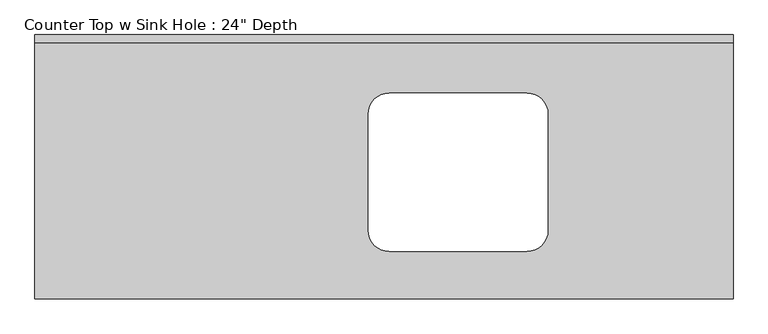
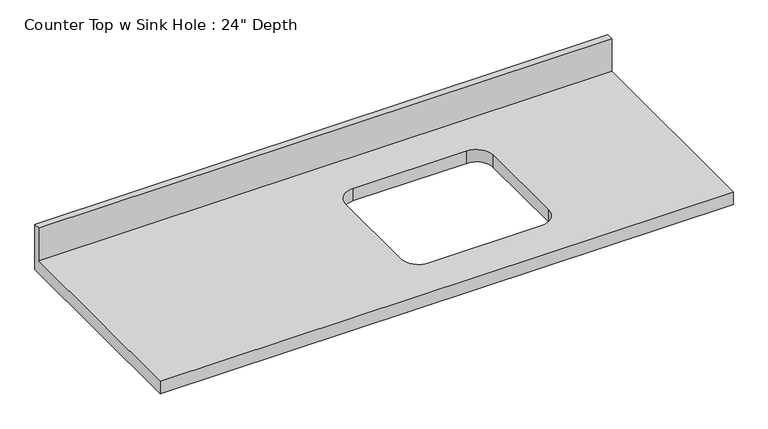
"""IFC4 building model written with IfcOpenShell, lengths in millimetres: furniture geometry."""

from ifc_helpers import new_model, si_unit, frame, origin, place, context, project, spatial, polyline, circle_curve, source, transform, mapped, element, save
from ifc_brep_helpers import plane_surface, revolved_surface, advanced_brep


def furniture_1781b5df(model_context):
    return source(origin(), model_context, "Body", "AdvancedBrep", [
        advanced_brep(
        [(-1200.4622951, -635.0, 914.4), (475.9377049, -635.0, 914.4), (475.9377049, -19.05, 914.4), (-1200.4622951, -19.05, 914.4), (-349.5622951, -139.7, 914.4), (-19.3622951, -139.7, 914.4), (31.4377049, -190.5, 914.4), (31.4377049, -469.9, 914.4), (-19.3622951, -520.7, 914.4), (-349.5622951, -520.7, 914.4), (-400.3622951, -469.9, 914.4), (-400.3622951, -190.5, 914.4), (475.9377049, 0.0, 876.3), (475.9377049, -635.0, 876.3), (-1200.4622951, -635.0, 876.3), (-1200.4622951, 0.0, 876.3), (-19.3622951, -139.7, 876.3), (-349.5622951, -139.7, 876.3), (-400.3622951, -190.5, 876.3), (-400.3622951, -469.9, 876.3), (-349.5622951, -520.7, 876.3), (-19.3622951, -520.7, 876.3), (31.4377049, -469.9, 876.3), (31.4377049, -190.5, 876.3), (-1200.4622951, 0.0, 1016.0), (475.9377049, 0.0, 1016.0), (-1200.4622951, -19.05, 1016.0), (475.9377049, -19.05, 1016.0)],
        [
            (0, 1),
            (1, 2),
            (2, 3),
            (3, 0),
            (4, 5),
            (5, 6, circle_curve(frame((-19.3622951, -190.5, 914.4), z_axis=(0.0, 0.0, -1.0), x_axis=(1.0, 0.0, 0.0)), 50.8)),
            (6, 7),
            (7, 8, circle_curve(frame((-19.3622951, -469.9, 914.4), z_axis=(0.0, 0.0, -1.0), x_axis=(1.0, 0.0, 0.0)), 50.8)),
            (8, 9),
            (9, 10, circle_curve(frame((-349.5622951, -469.9, 914.4), z_axis=(0.0, 0.0, -1.0), x_axis=(1.0, 0.0, 0.0)), 50.8)),
            (10, 11),
            (11, 4, circle_curve(frame((-349.5622951, -190.5, 914.4), z_axis=(0.0, 0.0, -1.0), x_axis=(1.0, 0.0, 0.0)), 50.8)),
            (12, 13),
            (13, 14),
            (14, 15),
            (15, 12),
            (16, 17),
            (17, 18, circle_curve(frame((-349.5622951, -190.5, 876.3), z_axis=(0.0, 0.0, 1.0), x_axis=(1.0, 0.0, 0.0)), 50.8)),
            (18, 19),
            (19, 20, circle_curve(frame((-349.5622951, -469.9, 876.3), z_axis=(0.0, 0.0, 1.0), x_axis=(1.0, 0.0, 0.0)), 50.8)),
            (20, 21),
            (21, 22, circle_curve(frame((-19.3622951, -469.9, 876.3), z_axis=(0.0, 0.0, 1.0), x_axis=(1.0, 0.0, 0.0)), 50.8)),
            (22, 23),
            (23, 16, circle_curve(frame((-19.3622951, -190.5, 876.3), z_axis=(0.0, 0.0, 1.0), x_axis=(1.0, 0.0, 0.0)), 50.8)),
            (15, 24),
            (24, 25),
            (25, 12),
            (14, 0),
            (3, 26),
            (26, 24),
            (13, 1),
            (25, 27),
            (27, 2),
            (4, 17),
            (16, 5),
            (11, 18),
            (10, 19),
            (9, 20),
            (8, 21),
            (7, 22),
            (6, 23),
            (26, 27),
        ],
        [
            plane_surface(frame((-1200.4622951, 0.0, 914.4), z_axis=(0.0, 0.0, 1.0), x_axis=(-1.0, 0.0, 0.0))),
            plane_surface(frame((-1200.4622951, 0.0, 876.3), z_axis=(0.0, 0.0, -1.0), x_axis=(1.0, 0.0, 0.0))),
            plane_surface(frame((475.9377049, 0.0, 914.4), z_axis=(0.0, 1.0, 0.0), x_axis=(0.0, 0.0, -1.0))),
            plane_surface(frame((-1200.4622951, 0.0, 914.4), z_axis=(-1.0, 0.0, 0.0), x_axis=(0.0, 0.0, -1.0))),
            plane_surface(frame((-1200.4622951, -635.0, 914.4), z_axis=(0.0, -1.0, 0.0), x_axis=(0.0, 0.0, -1.0))),
            plane_surface(frame((475.9377049, -635.0, 914.4), z_axis=(1.0, 0.0, 0.0), x_axis=(0.0, 0.0, -1.0))),
            plane_surface(frame((-19.3622951, -139.7, 914.4), z_axis=(0.0, -1.0, 0.0), x_axis=(0.0, 0.0, -1.0))),
            revolved_surface(polyline([(-298.76229509999996, -190.5, 914.4), (-298.76229509999996, -190.5, 876.3)]), (-349.5622951, -190.5, 876.3), (0.0, 0.0, 1.0)),
            plane_surface(frame((-400.3622951, -190.5, 914.4), z_axis=(1.0, 0.0, 0.0), x_axis=(0.0, 0.0, -1.0))),
            revolved_surface(polyline([(-298.76229509999996, -469.9, 914.4), (-298.76229509999996, -469.9, 876.3)]), (-349.5622951, -469.9, 876.3), (0.0, 0.0, 1.0)),
            plane_surface(frame((-349.5622951, -520.7, 914.4), z_axis=(0.0, 1.0, 0.0), x_axis=(0.0, 0.0, -1.0))),
            revolved_surface(polyline([(31.437704899999996, -469.9, 914.4), (31.437704899999996, -469.9, 876.3)]), (-19.3622951, -469.9, 876.3), (0.0, 0.0, 1.0)),
            plane_surface(frame((31.4377049, -469.9, 914.4), z_axis=(-1.0, 0.0, 0.0), x_axis=(0.0, 0.0, -1.0))),
            revolved_surface(polyline([(31.437704899999996, -190.5, 914.4), (31.437704899999996, -190.5, 876.3)]), (-19.3622951, -190.5, 876.3), (0.0, 0.0, 1.0)),
            plane_surface(frame((-1200.4622951, 0.0, 1016.0), z_axis=(0.0, 0.0, 1.0), x_axis=(0.0, -1.0, 0.0))),
            plane_surface(frame((-1200.4622951, -19.05, 1016.0), z_axis=(0.0, -1.0, 0.0), x_axis=(0.0, 0.0, -1.0))),
        ],
        [
            (0, [[1, 2, 3, 4], [5, 6, 7, 8, 9, 10, 11, 12]]),
            (1, [[13, 14, 15, 16], [17, 18, 19, 20, 21, 22, 23, 24]]),
            (2, [[-16, 25, 26, 27]]),
            (3, [[-15, 28, -4, 29, 30, -25]]),
            (4, [[-1, -28, -14, 31]]),
            (5, [[-13, -27, 32, 33, -2, -31]]),
            (6, [[34, -17, 35, -5]]),
            (7, [[-34, -12, 36, -18]]),
            (8, [[-36, -11, 37, -19]]),
            (9, [[-37, -10, 38, -20]]),
            (10, [[-38, -9, 39, -21]]),
            (11, [[-39, -8, 40, -22]]),
            (12, [[-40, -7, 41, -23]]),
            (13, [[-35, -24, -41, -6]]),
            (14, [[-30, 42, -32, -26]]),
            (15, [[-42, -29, -3, -33]]),
        ],
    ),
    ])


if __name__ == "__main__":
    model = new_model("IFC4")
    model_context = context("Model", 3, world=origin())
    ifc_project = project(units=[si_unit("LENGTHUNIT", "METRE", prefix="MILLI")], contexts=[model_context])
    site = spatial("IfcSite", under=ifc_project)
    building = spatial("IfcBuilding", under=site)
    placement = place(None, origin())
    furniture_shape = furniture_1781b5df(model_context)
    element("IfcFurniture", 1, ObjectType="Counter Top w Sink Hole : 24\" Depth", at=placement, inside=building, context=model_context, shape_type="MappedRepresentation", body=[
        mapped(furniture_shape, transform((0.0, 0.0, 0.0), x_axis=(1.0, 0.0, 0.0), y_axis=(0.0, 1.0, 0.0), z_axis=(0.0, 0.0, 1.0))),
    ])
    save(model, "model.ifc")

# Revit data of these elements
# Type "Counter Top w Sink Hole : 24\" Depth"
#   Assembly Code = "C1030400"
#   Counter Thickness = 0' - 1 1/2"
#   Depth = 2' - 1"
#   Height = 3' - 0"
#   Length [instance default] = 8' - 0"
#   Sink Location [instance default] = 2' - 0"
#   Sink Location To Wall [instance default] = 0' - 6"
#   Sink Opening Depth [instance default] = 1' - 3"
#   Sink Opening Width [instance default] = 2' - 3"
#   Counter Top Material = none
#   Default Elevation = 0
# Element 1 (IfcFurniture, "Counter Top w Sink Hole : 24\" Depth")
#   Length = 5' - 6"
#   Sink Location = 3' - 4"
#   Sink Opening Depth = 1' - 2"
#   Sink Opening Width = 1' - 4"
#   Materials on its faces: "Counter Top"
# Materials
#   "Counter Top": class "Wood", colour RGB 226 177 128, transparency 0
